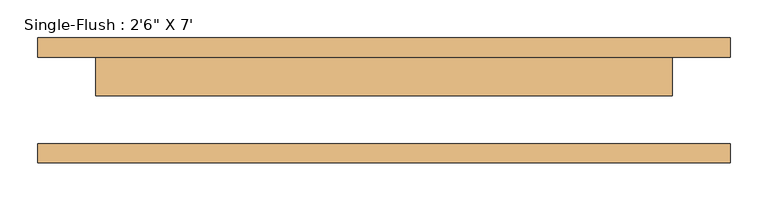
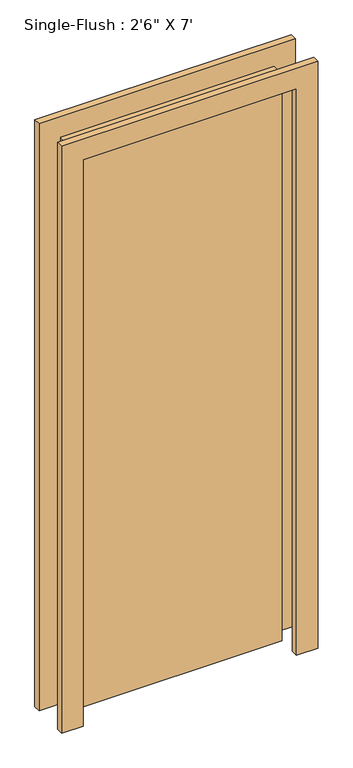
"""IFC4 building model written with IfcOpenShell, lengths in millimetres: door geometry."""

from ifc_helpers import new_model, si_unit, frame, origin, origin_with_axes, place, context, project, spatial, polyline, outline, extrude, source, transform, mapped, element, save


def door_214872d5(model_context):
    return source(origin(), model_context, "Body", "SweptSolid", [
        extrude(outline(polyline([(2209.8, -457.2), (0.0, -457.2), (0.0, -381.0), (2133.6, -381.0), (2133.6, 381.0), (0.0, 381.0), (0.0, 457.2), (2209.8, 457.2), (2209.8, -457.2)])), frame((0.0, 57.15, 0.0), z_axis=(0.0, 1.0, 0.0), x_axis=(0.0, 0.0, 1.0)), (0.0, 0.0, 1.0), 25.4),
        extrude(outline(polyline([(2209.8, 457.2), (2209.8, -457.2), (0.0, -457.2), (0.0, -381.0), (2133.6, -381.0), (2133.6, 381.0), (0.0, 381.0), (0.0, 457.2), (2209.8, 457.2)])), frame((0.0, -82.55, 0.0), z_axis=(0.0, 1.0, 0.0), x_axis=(0.0, 0.0, 1.0)), (0.0, 0.0, 1.0), 25.4),
        extrude(outline(polyline([(381.0, 6.35), (-381.0, 6.35), (-381.0, 57.15), (381.0, 57.15), (381.0, 6.35)])), origin_with_axes(), (0.0, 0.0, 1.0), 2133.6),
    ])


if __name__ == "__main__":
    model = new_model("IFC4")
    model_context = context("Model", 3, world=origin())
    ifc_project = project(units=[si_unit("LENGTHUNIT", "METRE", prefix="MILLI")], contexts=[model_context])
    site = spatial("IfcSite", under=ifc_project)
    building = spatial("IfcBuilding", under=site)
    placement = place(None, origin())
    door_shape = door_214872d5(model_context)
    element("IfcDoor", 1, ObjectType="Single-Flush : 2'6\" X 7'", at=placement, inside=building, context=model_context, shape_type="MappedRepresentation", body=[
        mapped(door_shape, transform((0.0, 0.0, 0.0), x_axis=(1.0, 0.0, 0.0), y_axis=(0.0, 1.0, 0.0), z_axis=(0.0, 0.0, 1.0))),
    ])
    save(model, "model.ifc")

# Revit data of these elements
# Type "Single-Flush : 2'6\" X 7'"
#   Type Mark = "14"
#   Construction Type Id = "MDOOR"
#   Assembly Code = "C1020"
#   Analytic Construction = "Metal"
#   Thickness = 0' - 2"
#   Heat Transfer Coefficient (U) = 0.651978 BTU/(h·ft²·°F)
#   Height = 7' - 0"
#   Trim Projection Ext = 0' - 1"
#   Trim Projection Int = 0' - 1"
#   Trim Width = 0' - 3"
#   Width = 2' - 6"
#   Define Thermal Properties by = 1
#   Door Material = Door - Panel
#   Frame Material = Door - Frame
#   Visual Light Transmittance = 0
#   Solar Heat Gain Coefficient = 0
#   Function = (empty or 0)
#   Wall Closure = (empty or 0)
# Element 1 (IfcDoor, "Single-Flush : 2'6\" X 7'")
#   Materials on its faces: "Door - Frame", "Door - Panel"
# Materials
#   "Door - Panel": class "Wood", colour RGB 210 159 95, transparency 0, Cost = 0
#   "Door - Frame": colour RGB 118 70 51, transparency 0, Cost = 0
